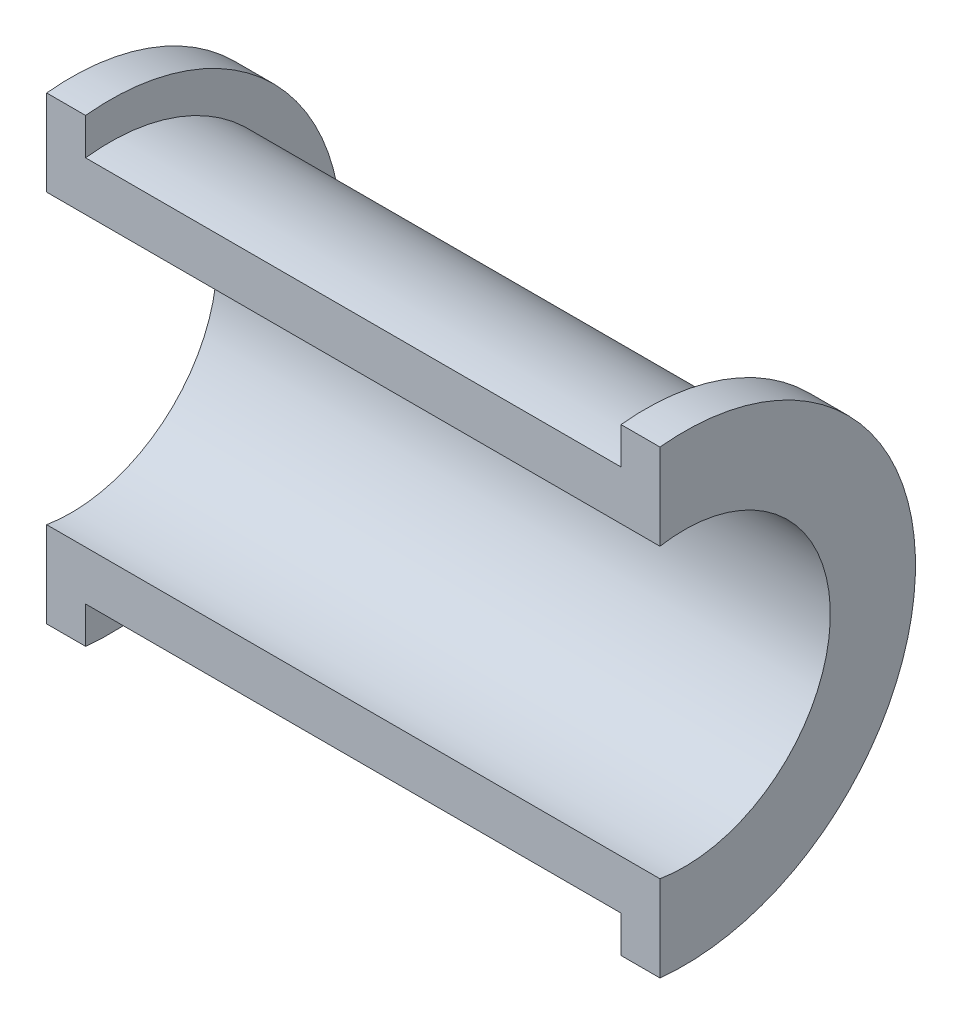
from build123d import *

# Parameters (mm, degrees)
HALF_SHELL_BODY_DEPTH   = 55
END_FLANGE_B_95X8_DEPTH = 8
END_START               = 8
END_FLANGE_A_95X8_DEPTH = 8
BORE_SKETCH_60_R        = 30
BORE_CUT_60_DEPTH       = 100


with BuildPart() as part:
    # Half Shell Profile Sketch → Half Shell Body (new, symmetric)
    with BuildSketch(Plane(origin=(0, 0, 0), x_dir=(0, 0, -1), z_dir=(1, 0, 0))):
        with BuildLine():
            Line((0, 39.686269666), (0, -39.686269666))
            ThreePointArc((0, -39.686269666), (45, 0), (0, 39.686269666))
        make_face()
    extrude(amount=HALF_SHELL_BODY_DEPTH, both=True)

    # End Flange B Sketch Ø95 → End Flange B Ø95x8 (add)
    with BuildSketch(Plane(origin=(55, 0, 0), x_dir=(0, 0, -1), z_dir=(1, 0, 0))):
        with BuildLine():
            Line((0, 47.236109069), (0, -47.236109069))
            ThreePointArc((0, -47.236109069), (52.5, 0), (0, 47.236109069))
        make_face()
    extrude(amount=END_FLANGE_B_95X8_DEPTH)

    # End Flange A Sketch Ø95 → End Flange A Ø95x8 (add)
    with BuildSketch(Plane.ZY.offset(55).offset(END_START)):
        with BuildLine():
            Line((0, 47.236109069), (0, -47.236109069))
            ThreePointArc((0, -47.236109069), (-52.5, 0), (0, 47.236109069))
        make_face()
    extrude(amount=-END_FLANGE_A_95X8_DEPTH)

    # Bore Sketch Ø60 → Bore Cut Ø60 (cut, symmetric)
    with BuildSketch(Plane(origin=(0, 0, 0), x_dir=(0, 0, -1), z_dir=(1, 0, 0))):
        with Locations((5, 0)):
            Circle(BORE_SKETCH_60_R)
    extrude(amount=BORE_CUT_60_DEPTH, both=True, mode=Mode.SUBTRACT)


solid = part.part
